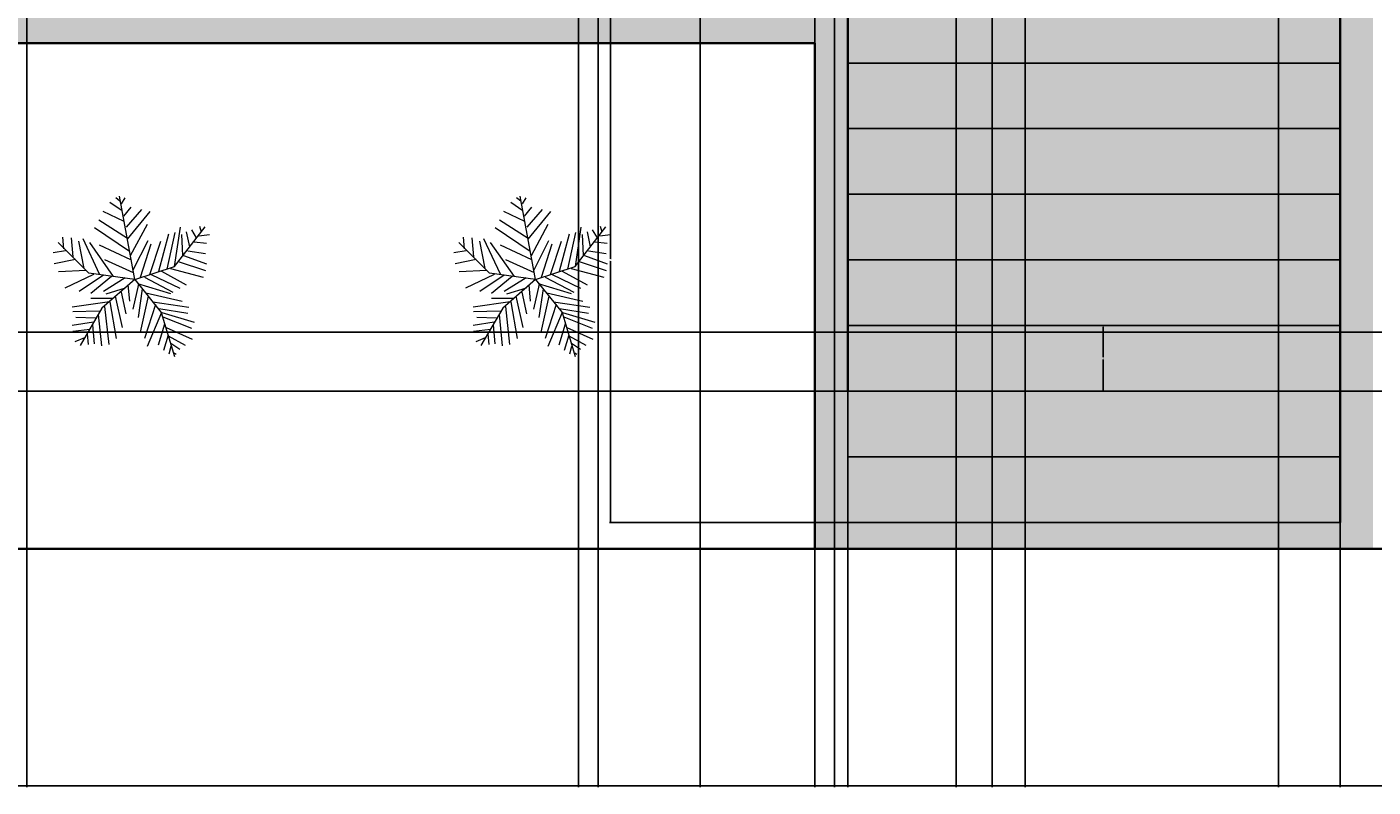
# Model space of a CAD drawing. Units: inches. Extents: x -7 to 546, y -27 to 766.
# Tile 2 of 9: x 127 to 332, y -27 to 89. Entities that reach past the tile are written whole.
import ezdxf

# ---------------------------------------------------------------- set-up
doc = ezdxf.new("R2010")
doc.units = ezdxf.units.IN
doc.header["$MEASUREMENT"] = 0
for name, color, linetype, lineweight in [('A-ANNO-DIMS', 2, 'Continuous', 18), ('A-FLOR-STRS', 7, 'Continuous', 25), ('A-WALL', 7, 'Continuous', 35), ('C-PROP', 7, 'Continuous', 35), ('L-PAVE', 7, 'Continuous', 18), ('L-PLNT', 94, 'Continuous', 18)]:
    doc.layers.add(name, color=color, linetype=linetype, lineweight=lineweight)
doc.layers.add('A-FLOR-PATT', color=143, linetype='Continuous', lineweight=13, true_color=0x7aafdf)
doc.layers.add('A-WALL-PATT', color=251, linetype='Continuous', lineweight=13, true_color=0x636466)
doc.styles.get("Standard").update_dxf_attribs({"font": 'arial.ttf'})
doc.dimstyles.get("Standard").update_dxf_attribs({"dimtxt": 0.18, "dimasz": 0.18, "dimexe": 0.18, "dimexo": 0.0625, "dimgap": 0.09, "dimtad": 0, "dimtih": 1, "dimtoh": 1, "dimdec": 4, "dimzin": 0, "dimdsep": 46, "dimtxsty": 'Standard', "dimcen": 0.09, "dimadec": 0, "dimazin": 0, "dimtfac": 1, "dimtdec": 4, "dimtofl": 0, "dimtmove": 0, "dimatfit": 3, "dimfxl": 1, "dimtolj": 1, "dimtzin": 0, "dimarcsym": 0})

# ---------------------------------------------------------------- blocks, each defined once
blk = doc.blocks.new('*U7')
for p, q in [((-10.186, 53.64), (-13.084, 55.962)), ((0, 0), (-10.5, 57)), ((-9.099, 51.782), (-6.563, 55.962)), ((-7.288, 39.707), (-21.778, 46.673)), ((-8.737, 47.138), (-17.069, 52.711)), ((-7.65, 43.423), (-2.578, 49.46)), ((-5.839, 35.992), (4.667, 48.067)), ((-5.114, 27.632), (10.463, 46.673)), ((-5.114, 28.097), (-24.676, 40.636)), ((-2.941, 16.486), (8.652, 37.85)), ((-48.585, 21.131), (-49.309, 29.026)), ((-43.513, 28.561), (-42.427, 15.558)), ((-35.544, 28.097), (-24.314, 3.947)), ((-3.665, 19.273), (-27.574, 35.527)), ((16.259, 5.805), (23.142, 31.348)), ((22.055, 7.198), (27.489, 32.277)), ((27, 9), (48, 36)), ((27.127, 9.056), (31.112, 35.992)), ((31.836, 30.883), (32.561, 16.486)), ((35.096, 32.741), (37.27, 22.524)), ((38.719, 34.134), (41.979, 28.561)), ((43.791, 29.954), (51.036, 30.883)), ((44.153, 36.456), (45.239, 32.741)), ((-47.498, 19.737), (-55.83, 18.344)), ((-31.5, 4.5), (-52.5, 25.5)), ((-38.442, 26.239), (-34.819, 7.663)), ((-14.533, 2.09), (-30.834, 25.31)), ((-24.314, 23.917), (-2.941, 13.7)), ((-1.129, 6.734), (9.014, 26.704)), ((3.942, 1.625), (11.187, 24.381)), ((10.101, 3.483), (17.708, 26.239)), ((36.183, 19.737), (48.137, 17.88)), ((40.53, 25.775), (48.862, 24.846)), ((-40.615, 13.7), (-55.105, 10.913)), ((-20.691, 13.7), (-1.129, 4.876)), ((29.662, 12.307), (48.137, 6.269)), ((33.285, 16.486), (48.862, 10.913)), ((-33.37, 6.269), (-52.207, 5.34)), ((-28.299, 3.483), (-47.86, -5.805)), ((-21.416, 3.018), (-38.079, -8.128)), ((0, 0), (-31.5, 4.5)), ((-15.982, 2.09), (-30.11, -9.521)), ((0, 0), (-22.5, -19.5)), ((-6.563, 1.161), (-21.416, -8.128)), ((0, 0), (27, 9)), ((0, 0), (18, -22.5)), ((6.478, 1.625), (26.04, -8.592)), ((11.187, 3.483), (30.749, -5.805)), ((18.07, 5.805), (35.096, -3.483)), ((24.229, 7.663), (46.688, 1.625)), ((-6.563, -5.805), (-19.967, -9.985)), ((-9.461, -8.592), (-6.201, -23.453)), ((-4.752, -3.483), (-3.665, -14.629)), ((2.493, -3.019), (-1.491, -20.202)), ((1.769, -2.555), (24.229, -9.521)), ((5.029, -6.27), (2.131, -25.775)), ((7.565, -9.056), (32.198, -14.629)), ((-17.431, -15.094), (-42.789, -18.809)), ((-15.257, -12.772), (-30.11, -12.772)), ((-20.691, -18.345), (-17.793, -44.352)), ((-17.069, -15.094), (-12.721, -40.172)), ((-13.446, -11.378), (-8.737, -32.741)), ((9.014, -11.378), (3.58, -35.992)), ((14.085, -16.951), (6.478, -40.172)), ((12.274, -15.094), (36.907, -18.809)), ((-24.314, -21.596), (-42.427, -22.06)), ((-26.849, -26.24), (-40.253, -25.775)), ((-22.5, -19.5), (-37.5, -45)), ((-25.038, -23.918), (-22.865, -45.281)), ((18.07, -22.524), (8.289, -45.745)), ((16.259, -19.738), (36.183, -22.989)), ((18, -22.5), (27, -52.5)), ((18.433, -22.524), (40.53, -29.026)), ((19.157, -25.311), (38.719, -33.206)), ((-28.299, -29.026), (-42.789, -31.348)), ((-30.834, -34.135), (-42.427, -35.528)), ((-29.023, -30.884), (-27.936, -43.887)), ((20.244, -30.419), (15.897, -44.816)), ((21.331, -32.741), (39.081, -40.636)), ((-34.457, -39.708), (-40.978, -42.494)), ((-32.646, -36.921), (-31.921, -44.352)), ((22.78, -37.85), (19.519, -48.532)), ((22.78, -38.314), (34.372, -44.816)), ((24.591, -45.745), (23.142, -50.854)), ((24.591, -43.423), (30.749, -47.603)), ((26.764, -49.925), (28.213, -50.854))]:
    blk.add_line(p, q)
blk = doc.blocks.new('*D30')
at = {"layer": 'A-ANNO-DIMS', "color": 0, "lineweight": -2, "transparency": 16777216}
for p, q in [((29.23, 9.68), (29.23, -26.56)), ((509.23, 9.68), (509.23, -26.56)), ((29.41, -26.38), (268.94, -26.38)), ((509.05, -26.38), (269.52, -26.38))]:
    blk.add_line(p, q, dxfattribs=at)
at = {"layer": 'A-ANNO-DIMS', "color": 0, "transparency": 16777216}
for points in [[(29.41, -26.35), (29.41, -26.41), (29.23, -26.38)], [(509.05, -26.35), (509.05, -26.41), (509.23, -26.38)]]:
    blk.add_solid(points, dxfattribs=at)
at = {"layer": 'Defpoints', "color": 0, "transparency": 16777216}
for p in [(29.23, 9.74), (509.23, 9.74), (509.23, -26.38)]:
    blk.add_point(p, dxfattribs=at)
at = {"layer": 'A-ANNO-DIMS', "color": 0, "transparency": 16777216, "insert": (269.23, -26.38), "char_height": 0.18, "attachment_point": 5}
blk.add_mtext('\\A1;480', dxfattribs=at)
blk = doc.blocks.new('*D39')
at = {"layer": 'A-ANNO-DIMS', "color": 0, "lineweight": -2, "transparency": 16777216}
for p, q in [((214.23, 600.68), (214.23, -26.56)), ((250.23, 600.68), (250.23, -26.56)), ((214.41, -26.38), (232.01, -26.38)), ((250.05, -26.38), (232.45, -26.38))]:
    blk.add_line(p, q, dxfattribs=at)
at = {"layer": 'A-ANNO-DIMS', "color": 0, "transparency": 16777216}
for points in [[(214.41, -26.35), (214.41, -26.41), (214.23, -26.38)], [(250.05, -26.35), (250.05, -26.41), (250.23, -26.38)]]:
    blk.add_solid(points, dxfattribs=at)
at = {"layer": 'Defpoints', "color": 0, "transparency": 16777216}
for p in [(214.23, 600.74), (250.23, 600.74), (250.23, -26.38)]:
    blk.add_point(p, dxfattribs=at)
at = {"layer": 'A-ANNO-DIMS', "color": 0, "transparency": 16777216, "insert": (232.23, -26.38), "char_height": 0.18, "attachment_point": 5}
blk.add_mtext('\\A1;36', dxfattribs=at)
blk = doc.blocks.new('*D41')
at = {"layer": 'A-ANNO-DIMS', "color": 0, "lineweight": -2, "transparency": 16777216}
for p, q in [((274.23, 600.68), (274.23, -26.56)), ((279.23, 600.68), (279.23, -26.56)), ((274.41, -26.38), (276.58, -26.38)), ((279.05, -26.38), (276.88, -26.38))]:
    blk.add_line(p, q, dxfattribs=at)
at = {"layer": 'A-ANNO-DIMS', "color": 0, "transparency": 16777216}
for points in [[(274.41, -26.35), (274.41, -26.41), (274.23, -26.38)], [(279.05, -26.35), (279.05, -26.41), (279.23, -26.38)]]:
    blk.add_solid(points, dxfattribs=at)
at = {"layer": 'Defpoints', "color": 0, "transparency": 16777216}
for p in [(274.23, 600.74), (279.23, 600.74), (279.23, -26.38)]:
    blk.add_point(p, dxfattribs=at)
at = {"layer": 'A-ANNO-DIMS', "color": 0, "transparency": 16777216, "insert": (276.73, -26.38), "char_height": 0.18, "attachment_point": 5}
blk.add_mtext('\\A1;5', dxfattribs=at)
blk = doc.blocks.new('*D42')
at = {"layer": 'A-ANNO-DIMS', "color": 0, "lineweight": -2, "transparency": 16777216}
for p, q in [((211.23, 696.68), (211.23, -26.56)), ((229.74, 696.68), (229.74, -26.56)), ((211.41, -26.38), (220.12, -26.38)), ((229.56, -26.38), (220.85, -26.38))]:
    blk.add_line(p, q, dxfattribs=at)
at = {"layer": 'A-ANNO-DIMS', "color": 0, "transparency": 16777216}
for points in [[(211.41, -26.35), (211.41, -26.41), (211.23, -26.38)], [(229.56, -26.35), (229.56, -26.41), (229.74, -26.38)]]:
    blk.add_solid(points, dxfattribs=at)
at = {"layer": 'Defpoints', "color": 0, "transparency": 16777216}
for p in [(211.23, 696.74), (229.74, 696.74), (229.74, -26.38)]:
    blk.add_point(p, dxfattribs=at)
at = {"layer": 'A-ANNO-DIMS', "color": 0, "transparency": 16777216, "insert": (220.49, -26.38), "char_height": 0.18, "attachment_point": 5}
blk.add_mtext('\\A1;18.51', dxfattribs=at)
blk = doc.blocks.new('*D43')
at = {"layer": 'A-ANNO-DIMS', "color": 0, "lineweight": -2, "transparency": 16777216}
for p, q in [((317.84, 696.68), (317.84, -26.56)), ((327.23, 696.68), (327.23, -26.56)), ((318.02, -26.38), (322.21, -26.38)), ((327.05, -26.38), (322.86, -26.38))]:
    blk.add_line(p, q, dxfattribs=at)
at = {"layer": 'A-ANNO-DIMS', "color": 0, "transparency": 16777216}
for points in [[(318.02, -26.35), (318.02, -26.41), (317.84, -26.38)], [(327.05, -26.35), (327.05, -26.41), (327.23, -26.38)]]:
    blk.add_solid(points, dxfattribs=at)
at = {"layer": 'Defpoints', "color": 0, "transparency": 16777216}
for p in [(317.84, 696.74), (327.23, 696.74), (327.23, -26.38)]:
    blk.add_point(p, dxfattribs=at)
at = {"layer": 'A-ANNO-DIMS', "color": 0, "transparency": 16777216, "insert": (322.54, -26.38), "char_height": 0.18, "attachment_point": 5}
blk.add_mtext('\\A1;9.39', dxfattribs=at)
blk = doc.blocks.new('*D45')
at = {"layer": 'A-ANNO-DIMS', "color": 0, "lineweight": -2, "transparency": 16777216}
for p, q in [((211.23, 600.68), (211.23, -26.56)), ((214.23, 600.68), (214.23, -26.56)), ((211.41, -26.38), (212.58, -26.38)), ((214.05, -26.38), (212.88, -26.38))]:
    blk.add_line(p, q, dxfattribs=at)
at = {"layer": 'A-ANNO-DIMS', "color": 0, "transparency": 16777216}
for points in [[(211.41, -26.35), (211.41, -26.41), (211.23, -26.38)], [(214.05, -26.35), (214.05, -26.41), (214.23, -26.38)]]:
    blk.add_solid(points, dxfattribs=at)
at = {"layer": 'Defpoints', "color": 0, "transparency": 16777216}
for p in [(211.23, 600.74), (214.23, 600.74), (214.23, -26.38)]:
    blk.add_point(p, dxfattribs=at)
at = {"layer": 'A-ANNO-DIMS', "color": 0, "transparency": 16777216, "insert": (212.73, -26.38), "char_height": 0.18, "attachment_point": 5}
blk.add_mtext('\\A1;3', dxfattribs=at)
blk = doc.blocks.new('*D49')
at = {"layer": 'A-ANNO-DIMS', "color": 0, "lineweight": -2, "transparency": 16777216}
for p, q in [((127.23, 91.68), (127.23, -26.56)), ((247.23, 91.68), (247.23, -26.56)), ((127.41, -26.38), (186.95, -26.38)), ((247.05, -26.38), (187.51, -26.38))]:
    blk.add_line(p, q, dxfattribs=at)
at = {"layer": 'A-ANNO-DIMS', "color": 0, "transparency": 16777216}
for points in [[(127.41, -26.35), (127.41, -26.41), (127.23, -26.38)], [(247.05, -26.35), (247.05, -26.41), (247.23, -26.38)]]:
    blk.add_solid(points, dxfattribs=at)
at = {"layer": 'Defpoints', "color": 0, "transparency": 16777216}
for p in [(127.23, 91.74), (247.23, 91.74), (247.23, -26.38)]:
    blk.add_point(p, dxfattribs=at)
at = {"layer": 'A-ANNO-DIMS', "color": 0, "transparency": 16777216, "insert": (187.23, -26.38), "char_height": 0.18, "attachment_point": 5}
blk.add_mtext('\\A1;120', dxfattribs=at)
blk = doc.blocks.new('*D55')
at = {"layer": 'A-ANNO-DIMS', "color": 0, "lineweight": -2, "transparency": 16777216}
for p, q in [((252.23, 13.68), (252.23, -26.56)), ((327.23, 13.68), (327.23, -26.56)), ((252.41, -26.38), (289.51, -26.38)), ((327.05, -26.38), (289.95, -26.38))]:
    blk.add_line(p, q, dxfattribs=at)
at = {"layer": 'A-ANNO-DIMS', "color": 0, "transparency": 16777216}
for points in [[(252.41, -26.35), (252.41, -26.41), (252.23, -26.38)], [(327.05, -26.35), (327.05, -26.41), (327.23, -26.38)]]:
    blk.add_solid(points, dxfattribs=at)
at = {"layer": 'Defpoints', "color": 0, "transparency": 16777216}
for p in [(252.23, 13.74), (327.23, 13.74), (252.23, -26.38)]:
    blk.add_point(p, dxfattribs=at)
at = {"layer": 'A-ANNO-DIMS', "color": 0, "transparency": 16777216, "insert": (289.73, -26.38), "char_height": 0.18, "attachment_point": 5}
blk.add_mtext('\\A1;75', dxfattribs=at)
blk = doc.blocks.new('*D61')
at = {"layer": 'A-ANNO-DIMS', "color": 0, "lineweight": -2, "transparency": 16777216}
for p, q in [((327.17, 43.74), (290.93, 43.74)), ((291.11, 43.56), (291.11, 38.93)), ((291.11, 33.92), (291.11, 38.56)), ((327.17, 33.74), (290.93, 33.74))]:
    blk.add_line(p, q, dxfattribs=at)
at = {"layer": 'A-ANNO-DIMS', "color": 0, "transparency": 16777216}
for points in [[(291.08, 43.56), (291.14, 43.56), (291.11, 43.74)], [(291.08, 33.92), (291.14, 33.92), (291.11, 33.74)]]:
    blk.add_solid(points, dxfattribs=at)
at = {"layer": 'Defpoints', "color": 0, "transparency": 16777216}
for p in [(291.11, 43.74), (327.23, 43.74), (327.23, 33.74)]:
    blk.add_point(p, dxfattribs=at)
at = {"layer": 'A-ANNO-DIMS', "color": 0, "transparency": 16777216, "insert": (291.11, 38.74), "char_height": 0.18, "attachment_point": 5}
blk.add_mtext('\\A1;10', dxfattribs=at)
blk = doc.blocks.new('*D65')
at = {"layer": 'A-ANNO-DIMS', "color": 0, "lineweight": -2, "transparency": 16777216}
for p, q in [((461.17, 42.74), (-7.07, 42.74)), ((-6.89, 42.56), (-6.89, 38.43)), ((-6.89, 33.92), (-6.89, 38.06)), ((461.17, 33.74), (-7.07, 33.74))]:
    blk.add_line(p, q, dxfattribs=at)
at = {"layer": 'A-ANNO-DIMS', "color": 0, "transparency": 16777216}
for points in [[(-6.92, 42.56), (-6.86, 42.56), (-6.89, 42.74)], [(-6.92, 33.92), (-6.86, 33.92), (-6.89, 33.74)]]:
    blk.add_solid(points, dxfattribs=at)
at = {"layer": 'Defpoints', "color": 0, "transparency": 16777216}
for p in [(-6.89, 42.74), (461.23, 42.74), (461.23, 33.74)]:
    blk.add_point(p, dxfattribs=at)
at = {"layer": 'A-ANNO-DIMS', "color": 0, "transparency": 16777216, "insert": (-6.89, 38.24), "char_height": 0.18, "attachment_point": 5}
blk.add_mtext('\\A1;9', dxfattribs=at)
blk = doc.blocks.new('*D66')
at = {"layer": 'A-ANNO-DIMS', "color": 0, "lineweight": -2, "transparency": 16777216}
for p, q in [((252.17, 93.74), (215.93, 93.74)), ((216.11, 93.56), (216.11, 53.93)), ((216.11, 13.92), (216.11, 53.56)), ((252.17, 13.74), (215.93, 13.74))]:
    blk.add_line(p, q, dxfattribs=at)
at = {"layer": 'A-ANNO-DIMS', "color": 0, "transparency": 16777216}
for points in [[(216.08, 93.56), (216.14, 93.56), (216.11, 93.74)], [(216.08, 13.92), (216.14, 13.92), (216.11, 13.74)]]:
    blk.add_solid(points, dxfattribs=at)
at = {"layer": 'Defpoints', "color": 0, "transparency": 16777216}
for p in [(216.11, 93.74), (252.23, 93.74), (252.23, 13.74)]:
    blk.add_point(p, dxfattribs=at)
at = {"layer": 'A-ANNO-DIMS', "color": 0, "transparency": 16777216, "insert": (216.11, 53.74), "char_height": 0.18, "attachment_point": 5}
blk.add_mtext('\\A1;80', dxfattribs=at)
blk = doc.blocks.new('*D85')
at = {"layer": 'A-ANNO-DIMS', "color": 0, "lineweight": -2, "transparency": 16777216}
for p, q in [((274.23, 696.68), (274.23, -26.56)), ((268.74, 692.17), (268.74, -26.56)), ((268.92, -26.38), (271.09, -26.38)), ((274.05, -26.38), (271.88, -26.38))]:
    blk.add_line(p, q, dxfattribs=at)
at = {"layer": 'A-ANNO-DIMS', "color": 0, "transparency": 16777216}
for points in [[(268.92, -26.35), (268.92, -26.41), (268.74, -26.38)], [(274.05, -26.35), (274.05, -26.41), (274.23, -26.38)]]:
    blk.add_solid(points, dxfattribs=at)
at = {"layer": 'Defpoints', "color": 0, "transparency": 16777216}
for p in [(274.23, 696.74), (268.74, 692.23), (268.74, -26.38)]:
    blk.add_point(p, dxfattribs=at)
at = {"layer": 'A-ANNO-DIMS', "color": 0, "transparency": 16777216, "insert": (271.49, -26.38), "char_height": 0.18, "attachment_point": 5}
blk.add_mtext('\\A1;5.493', dxfattribs=at)

msp = doc.modelspace()

# ---------------------------------------------------------------- hatches: boundary and pattern name
at = {"layer": 'A-FLOR-PATT'}
h = msp.add_hatch(color=256, dxfattribs=at)
h.dxf.hatch_style = 1
h.paths.add_polyline_path([(327.2319, 93.744), (252.2319, 93.744), (252.2319, 83.744), (327.2319, 83.744)])
h.paths.add_polyline_path([(327.2319, 83.744), (252.2319, 83.744), (252.2319, 73.744), (327.2319, 73.744)])
h.paths.add_polyline_path([(327.2319, 73.744), (252.2319, 73.744), (252.2319, 63.744), (327.2319, 63.744)])
h.paths.add_polyline_path([(327.2319, 63.744), (252.2319, 63.744), (252.2319, 53.744), (327.2319, 53.744)])
h.paths.add_polyline_path([(327.2319, 53.744), (252.2319, 53.744), (252.2319, 43.744), (327.2319, 43.744)])
h.paths.add_polyline_path([(327.2319, 43.744), (252.2319, 43.744), (252.2319, 33.744), (327.2319, 33.744)])
h.paths.add_polyline_path([(327.2319, 33.744), (252.2319, 33.744), (252.2319, 23.744), (327.2319, 23.744)])
h.paths.add_polyline_path([(327.2319, 23.744), (252.2319, 23.744), (252.2319, 13.744), (327.2319, 13.744)])
h = msp.add_hatch(color=256, dxfattribs=at)
h.dxf.hatch_style = 1
h.paths.add_polyline_path([(252.2319, 33.744), (247.2319, 33.744), (247.2319, 9.744), (332.2319, 9.744), (332.2319, 33.744), (327.2319, 33.744), (327.2319, 13.744), (252.2319, 13.744)])
at = {"layer": 'A-WALL-PATT'}
h = msp.add_hatch(color=256, dxfattribs=at)
h.dxf.hatch_style = 1
h.paths.add_polyline_path([(62.2319, 696.744), (86.6896, 696.744), (86.6896, 705.744), (53.2319, 705.744), (53.2319, 627.8642), (57.7271, 627.8642), (62.2319, 627.8642)])
h.paths.add_polyline_path([(229.7414, 705.744), (134.6896, 705.744), (134.6896, 696.744), (206.2319, 696.744), (206.2319, 567.744), (211.2319, 567.744), (211.2319, 595.744), (214.2319, 595.744), (214.2319, 600.744), (211.2319, 600.744), (211.2319, 696.744), (229.7414, 696.744)])
h.paths.add_polyline_path([(293.8423, 705.744), (253.7414, 705.744), (253.7414, 696.744), (274.2319, 696.744), (274.2319, 600.744), (279.2319, 600.744), (279.2319, 696.744), (293.8423, 696.744)])
h.paths.add_polyline_path([(393.9743, 705.744), (317.8423, 705.744), (317.8423, 696.744), (327.2319, 696.744), (327.2319, 651.744), (332.2319, 651.744), (332.2319, 696.744), (393.9743, 696.744)])
h.paths.add_polyline_path([(485.2319, 705.744), (441.9743, 705.744), (441.9743, 696.744), (476.2319, 696.744), (476.2319, 663.6898), (480.7319, 663.6898), (485.2319, 663.6898)])
h.paths.add_polyline_path([(485.2319, 615.6898), (476.2319, 615.6898), (476.2319, 528.744), (332.2319, 528.744), (332.2319, 531.744), (327.2319, 531.744), (327.2319, 523.744), (375.2319, 523.744), (375.2319, 427.744), (327.2319, 427.744), (327.2319, 419.744), (332.2319, 419.744), (332.2319, 422.744), (413.089, 422.744), (413.089, 427.744), (380.2319, 427.744), (380.2319, 523.744), (476.2319, 523.744), (476.2319, 490.9334), (485.2319, 490.9334)])
h.paths.add_polyline_path([(485.2319, 466.9334), (476.2319, 466.9334), (476.2319, 370.0932), (480.7319, 370.0932), (485.2319, 370.0932)])
h.paths.add_polyline_path([(485.2319, 322.0932), (476.2319, 322.0932), (476.2319, 278.744), (332.2319, 278.744), (332.2319, 383.744), (327.2319, 383.744), (327.2319, 273.744), (327.2319, 270.744), (332.2319, 270.744), (332.2319, 273.744), (476.2319, 273.744), (476.2319, 201.0338), (480.7319, 201.0338), (485.2319, 201.0338)])
h.paths.add_polyline_path([(485.2319, 153.0338), (476.2319, 153.0338), (476.2319, 42.744), (461.2319, 42.744), (461.2319, 33.744), (485.2319, 33.744)])
h.paths.add_polyline_path([(332.2319, 234.744), (327.2319, 234.744), (327.2319, 160.744), (315.2319, 160.744), (315.2319, 151.744), (327.2319, 151.744), (327.2319, 33.744), (332.2319, 33.744)])
h.paths.add_polyline_path([(252.2319, 151.744), (258.4464, 151.744), (264.2319, 151.744), (264.2319, 160.744), (252.2319, 160.744), (252.2319, 172.744), (247.2319, 172.744), (247.2319, 91.744), (127.2319, 91.744), (127.2319, 196.744), (122.2319, 196.744), (122.2319, 91.744), (62.2319, 91.744), (62.2319, 126.1124), (53.2319, 126.1124), (53.2319, 9.744), (62.2319, 9.744), (62.2319, 86.744), (247.2319, 86.744), (247.2319, 33.744), (252.2319, 33.744), (252.2319, 53.744)])
h.paths.add_polyline_path([(62.2319, 235.744), (122.2319, 235.744), (122.2319, 232.744), (127.2319, 232.744), (127.2319, 235.744), (247.2319, 235.744), (247.2319, 220.744), (252.2319, 220.744), (252.2319, 240.744), (250.6678, 240.744), (247.2319, 240.744), (62.2319, 240.744), (62.2319, 322.0932), (53.2319, 322.0932), (53.2319, 174.1124), (57.7271, 174.1124), (62.2319, 174.1124)])

# ---------------------------------------------------------------- linework, layer by layer
at = {"layer": 'A-FLOR-STRS'}
for p, q in [((252.2319, 83.744), (327.2319, 83.744)), ((252.2319, 73.744), (327.2319, 73.744)), ((252.2319, 63.744), (327.2319, 63.744)), ((252.2319, 13.744), (252.2319, 53.744)), ((252.2319, 53.744), (327.2319, 53.744)), ((252.2319, 43.744), (327.2319, 43.744)), ((252.2319, 33.744), (327.2319, 33.744)), ((252.2319, 23.744), (327.2319, 23.744)), ((252.2319, 13.744), (327.2319, 13.744))]:
    msp.add_line(p, q, dxfattribs=at)
at = {"layer": 'A-WALL'}
for p, q in [((252.2319, 151.744), (252.2319, 33.744)), ((327.2319, 13.744), (327.2319, 151.744)), ((247.2319, 86.744), (62.2319, 86.744)), ((247.2319, 86.744), (247.2319, 9.744))]:
    msp.add_line(p, q, dxfattribs=at)
at = {"layer": 'C-PROP'}
msp.add_lwpolyline([(29.2319, 9.744), (509.2319, 9.744), (509.2319, 729.744), (29.2319, 729.744)], close=True, dxfattribs=at)
at = {"layer": 'L-PAVE'}
msp.add_lwpolyline([(247.2319, 33.744), (332.2319, 33.744)], dxfattribs=at)

# ---------------------------------------------------------------- block references
at = {"layer": 'L-PLNT', "xscale": 0.2228533388545292, "yscale": 0.2228533388545292, "zscale": 0.2228533388545292}
for p in [(143.6738, 50.7409), (204.7053, 50.7409)]:
    msp.add_blockref('*U7', p, dxfattribs=at)

# ---------------------------------------------------------------- dimensions: what is measured, and where the dimension line sits
at = {"layer": 'A-ANNO-DIMS'}
for base, p1, p2, override, picture, middle in [((229.7414, -26.381), (211.2319, 696.744), (229.7414, 696.744), {"dimdec": 2, "dimlfac": 1, "dimrnd": 0, "dimzin": 0, "dimdsep": 46, "dimlunit": 2}, '*D42', (220.4867, -26.381)), ((268.7385, -26.381), (274.2319, 696.744), (268.7385, 692.2322), {"dimdec": 3, "dimlfac": 1, "dimrnd": 0, "dimzin": 0, "dimdsep": 46, "dimlunit": 2}, '*D85', (271.4852, -26.381)), ((327.2319, -26.381), (317.8423, 696.744), (327.2319, 696.744), {"dimdec": 2, "dimlfac": 1, "dimrnd": 0, "dimzin": 0, "dimdsep": 46, "dimlunit": 2}, '*D43', (322.5371, -26.381)), ((214.2319, -26.381), (211.2319, 600.744), (214.2319, 600.744), {"dimdec": 0, "dimlfac": 1, "dimrnd": 0, "dimzin": 0, "dimdsep": 46, "dimlunit": 2}, '*D45', (212.7319, -26.381)), ((250.2319, -26.381), (214.2319, 600.744), (250.2319, 600.744), {"dimdec": 0, "dimlfac": 1, "dimrnd": 0, "dimzin": 0, "dimdsep": 46, "dimlunit": 2}, '*D39', (232.2319, -26.381)), ((279.2319, -26.381), (274.2319, 600.744), (279.2319, 600.744), {"dimdec": 0, "dimlfac": 1, "dimrnd": 0, "dimzin": 0, "dimdsep": 46, "dimlunit": 2}, '*D41', (276.7319, -26.381)), ((247.2319, -26.381), (127.2319, 91.744), (247.2319, 91.744), {"dimdec": 0, "dimlfac": 1, "dimrnd": 0, "dimzin": 0, "dimdsep": 46, "dimlunit": 2}, '*D49', (187.2319, -26.381)), ((252.2319, -26.381), (327.2319, 13.744), (252.2319, 13.744), {"dimdec": 0, "dimlfac": 1, "dimrnd": 0, "dimzin": 0, "dimdsep": 46, "dimlunit": 2}, '*D55', (289.7319, -26.381)), ((509.2319, -26.381), (29.2319, 9.744), (509.2319, 9.744), {"dimdec": 0, "dimlfac": 1, "dimrnd": 0, "dimzin": 0, "dimdsep": 46, "dimlunit": 2}, '*D30', (269.2319, -26.381))]:
    dim = msp.add_linear_dim(base=base, p1=p1, p2=p2, dimstyle='Standard', override=override, dxfattribs=at)
    dim.commit()
    dim.dimension.update_dxf_attribs({"geometry": picture, "text_midpoint": middle})
for base, p1, p2, picture, middle in [((216.1069, 93.744), (252.2319, 13.744), (252.2319, 93.744), '*D66', (216.1069, 53.744)), ((291.1069, 43.744), (327.2319, 33.744), (327.2319, 43.744), '*D61', (291.1069, 38.744)), ((-6.8931, 42.744), (461.2319, 33.744), (461.2319, 42.744), '*D65', (-6.8931, 38.244))]:
    dim = msp.add_linear_dim(base=base, p1=p1, p2=p2, angle=90, dimstyle='Standard', override={"dimdec": 0, "dimlfac": 1, "dimrnd": 0, "dimzin": 0, "dimdsep": 46, "dimlunit": 2}, dxfattribs=at)
    dim.commit()
    dim.dimension.update_dxf_attribs({"geometry": picture, "text_midpoint": middle})

doc.saveas('drawing.dxf')
